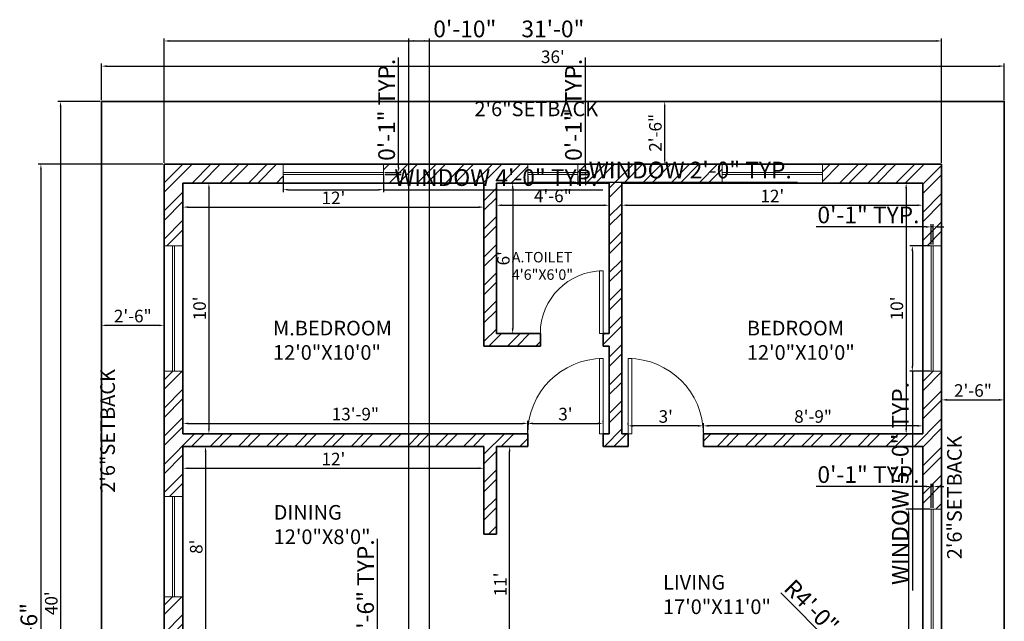
# Model space of a CAD drawing. Units: inches. Extents: x 4732 to 5926, y 2665 to 3255.
# Tile 8 of 8: x 5425 to 5896, y 2967 to 3255. Entities that reach past the tile are written whole.
import ezdxf

# ---------------------------------------------------------------- set-up
doc = ezdxf.new("R2010")
doc.units = ezdxf.units.IN
for name, color, linetype, lineweight in [('A-ANNO-DIMS', 2, 'Continuous', 18), ('A-ANNO-TEXT', 7, 'Continuous', 18), ('A-AREA-IDEN', 7, 'Continuous', 18), ('A-DOOR', 3, 'Continuous', 18), ('A-GLAZ', 4, 'Continuous', 18), ('A-WALL', 7, 'Continuous', 35), ('A-WALL-PATT', 8, 'Continuous', 13), ('C-PROP', 7, 'Continuous', 35)]:
    doc.layers.add(name, color=color, linetype=linetype, lineweight=lineweight)
doc.styles.get("Standard").update_dxf_attribs({"font": 'arial.ttf'})
doc.dimstyles.new('ISO-25', dxfattribs={"dimtxt": 8, "dimasz": 2.5, "dimexe": 1.25, "dimexo": 0.625, "dimtad": 1, "dimdec": 1, "dimlunit": 3, "dimtxsty": 'Standard', "dimcen": 2.5, "dimadec": 0, "dimazin": 0, "dimtfac": 1, "dimtdec": 1, "dimtmove": 0, "dimatfit": 3, "dimfxl": 1, "dimarcsym": 0})

# ---------------------------------------------------------------- blocks, each defined once
blk = doc.blocks.new('*U19')
for p, q in [((0, 0), (0, -6)), ((30, 0), (30, -6))]:
    blk.add_line(p, q)
blk.add_lwpolyline([(0, 0), (0, 30), (1.75, 30), (1.75, 0)], close=True)
blk.add_arc((0, 0), 30, 0, 90)
blk = doc.blocks.new('*U20')
for p, q in [((0, 0), (0, -6)), ((36, 0), (36, -6))]:
    blk.add_line(p, q)
blk.add_lwpolyline([(0, 0), (0, 36), (1.75, 36), (1.75, 0)], close=True)
blk.add_arc((0, 0), 36, 0, 90)
blk = doc.blocks.new('*D29')
at = {"layer": 'A-ANNO-DIMS', "color": 0, "lineweight": -2, "transparency": 16777216}
for p, q in [((5463.94, 3216.56), (5463.94, 3234.09)), ((5466.44, 3232.84), (5893.44, 3232.84)), ((5895.94, 3216.56), (5895.94, 3234.09))]:
    blk.add_line(p, q, dxfattribs=at)
at = {"layer": 'A-ANNO-DIMS', "color": 0, "transparency": 16777216}
for points in [[(5466.44, 3233.25), (5466.44, 3232.42), (5463.94, 3232.84)], [(5893.44, 3233.25), (5893.44, 3232.42), (5895.94, 3232.84)]]:
    blk.add_solid(points, dxfattribs=at)
at = {"layer": 'Defpoints', "color": 0, "transparency": 16777216}
for p in [(5895.94, 3232.84), (5463.94, 3215.93), (5895.94, 3215.93)]:
    blk.add_point(p, dxfattribs=at)
at = {"layer": 'A-ANNO-DIMS', "color": 0, "transparency": 16777216, "insert": (5679.94, 3236.53), "char_height": 6, "attachment_point": 5}
blk.add_mtext("36'", dxfattribs=at)
blk = doc.blocks.new('*D30')
at = {"layer": 'A-ANNO-DIMS', "color": 0, "lineweight": -2, "transparency": 16777216}
for p, q in [((5463.31, 3215.93), (5443.14, 3215.93)), ((5444.39, 3213.43), (5444.39, 2738.43)), ((5463.31, 2735.93), (5443.14, 2735.93))]:
    blk.add_line(p, q, dxfattribs=at)
at = {"layer": 'A-ANNO-DIMS', "color": 0, "transparency": 16777216}
for points in [[(5443.98, 3213.43), (5444.81, 3213.43), (5444.39, 3215.93)], [(5443.98, 2738.43), (5444.81, 2738.43), (5444.39, 2735.93)]]:
    blk.add_solid(points, dxfattribs=at)
at = {"layer": 'Defpoints', "color": 0, "transparency": 16777216}
for p in [(5463.94, 3215.93), (5444.39, 2735.93), (5463.94, 2735.93)]:
    blk.add_point(p, dxfattribs=at)
at = {"layer": 'A-ANNO-DIMS', "color": 0, "transparency": 16777216, "insert": (5440.71, 2975.93), "char_height": 6, "attachment_point": 5, "rotation": 90}
blk.add_mtext("40'", dxfattribs=at)
blk = doc.blocks.new('*D35')
at = {"layer": 'A-ANNO-DIMS', "color": 0, "lineweight": -2, "transparency": 16777216}
for p, q in [((5503.56, 3050.93), (5515.02, 3050.93)), ((5513.77, 3048.43), (5513.77, 2957.43)), ((5503.56, 2954.93), (5515.02, 2954.93))]:
    blk.add_line(p, q, dxfattribs=at)
at = {"layer": 'A-ANNO-DIMS', "color": 0, "transparency": 16777216}
for points in [[(5513.36, 3048.43), (5514.19, 3048.43), (5513.77, 3050.93)], [(5513.36, 2957.43), (5514.19, 2957.43), (5513.77, 2954.93)]]:
    blk.add_solid(points, dxfattribs=at)
at = {"layer": 'Defpoints', "color": 0, "transparency": 16777216}
for p in [(5502.94, 3050.93), (5502.94, 2954.93), (5513.77, 2954.93)]:
    blk.add_point(p, dxfattribs=at)
at = {"layer": 'A-ANNO-DIMS', "color": 0, "transparency": 16777216, "insert": (5510.08, 3002.93), "char_height": 6, "attachment_point": 5, "rotation": 90}
blk.add_mtext("8'", dxfattribs=at)
blk = doc.blocks.new('*D36')
at = {"layer": 'A-ANNO-DIMS', "color": 0, "lineweight": -2, "transparency": 16777216}
for p, q in [((5502.94, 3050.31), (5502.94, 3039.22)), ((5646.94, 3050.31), (5646.94, 3039.22)), ((5505.44, 3040.47), (5644.44, 3040.47))]:
    blk.add_line(p, q, dxfattribs=at)
at = {"layer": 'A-ANNO-DIMS', "color": 0, "transparency": 16777216}
for points in [[(5505.44, 3040.89), (5505.44, 3040.06), (5502.94, 3040.47)], [(5644.44, 3040.89), (5644.44, 3040.06), (5646.94, 3040.47)]]:
    blk.add_solid(points, dxfattribs=at)
at = {"layer": 'Defpoints', "color": 0, "transparency": 16777216}
for p in [(5502.94, 3050.93), (5646.94, 3050.93), (5646.94, 3040.47)]:
    blk.add_point(p, dxfattribs=at)
at = {"layer": 'A-ANNO-DIMS', "color": 0, "transparency": 16777216, "insert": (5574.94, 3044.11), "char_height": 6, "attachment_point": 5}
blk.add_mtext("12'", dxfattribs=at)
blk = doc.blocks.new('*D38')
at = {"layer": 'A-ANNO-DIMS', "color": 0, "lineweight": -2, "transparency": 16777216}
for p, q in [((5653.56, 3050.93), (5660.5, 3050.93)), ((5659.25, 2921.43), (5659.25, 3048.43)), ((5653.56, 2918.93), (5660.5, 2918.93))]:
    blk.add_line(p, q, dxfattribs=at)
at = {"layer": 'A-ANNO-DIMS', "color": 0, "transparency": 16777216}
for points in [[(5658.83, 3048.43), (5659.67, 3048.43), (5659.25, 3050.93)], [(5658.83, 2921.43), (5659.67, 2921.43), (5659.25, 2918.93)]]:
    blk.add_solid(points, dxfattribs=at)
at = {"layer": 'Defpoints', "color": 0, "transparency": 16777216}
for p in [(5652.94, 3050.93), (5659.25, 3050.93), (5652.94, 2918.93)]:
    blk.add_point(p, dxfattribs=at)
at = {"layer": 'A-ANNO-DIMS', "color": 0, "transparency": 16777216, "insert": (5655.61, 2984.93), "char_height": 6, "attachment_point": 5, "rotation": 90}
blk.add_mtext("11'", dxfattribs=at)
blk = doc.blocks.new('*D39')
at = {"layer": 'A-ANNO-DIMS', "color": 0, "lineweight": -2, "transparency": 16777216}
for p, q in [((5712.94, 3176.31), (5712.94, 3165.05)), ((5856.94, 3176.31), (5856.94, 3165.05)), ((5715.44, 3166.3), (5854.44, 3166.3))]:
    blk.add_line(p, q, dxfattribs=at)
at = {"layer": 'A-ANNO-DIMS', "color": 0, "transparency": 16777216}
for points in [[(5715.44, 3166.72), (5715.44, 3165.89), (5712.94, 3166.3)], [(5854.44, 3166.72), (5854.44, 3165.89), (5856.94, 3166.3)]]:
    blk.add_solid(points, dxfattribs=at)
at = {"layer": 'Defpoints', "color": 0, "transparency": 16777216}
for p in [(5712.94, 3176.93), (5856.94, 3176.93), (5856.94, 3166.3)]:
    blk.add_point(p, dxfattribs=at)
at = {"layer": 'A-ANNO-DIMS', "color": 0, "transparency": 16777216, "insert": (5784.94, 3169.94), "char_height": 6, "attachment_point": 5}
blk.add_mtext("12'", dxfattribs=at)
blk = doc.blocks.new('*D40')
at = {"layer": 'A-ANNO-DIMS', "color": 0, "lineweight": -2, "transparency": 16777216}
for p, q in [((5856.31, 3176.93), (5847.73, 3176.93)), ((5848.98, 3174.43), (5848.98, 3059.43)), ((5856.31, 3056.93), (5847.73, 3056.93))]:
    blk.add_line(p, q, dxfattribs=at)
at = {"layer": 'A-ANNO-DIMS', "color": 0, "transparency": 16777216}
for points in [[(5848.56, 3174.43), (5849.4, 3174.43), (5848.98, 3176.93)], [(5848.56, 3059.43), (5849.4, 3059.43), (5848.98, 3056.93)]]:
    blk.add_solid(points, dxfattribs=at)
at = {"layer": 'Defpoints', "color": 0, "transparency": 16777216}
for p in [(5856.94, 3176.93), (5848.98, 3056.93), (5856.94, 3056.93)]:
    blk.add_point(p, dxfattribs=at)
at = {"layer": 'A-ANNO-DIMS', "color": 0, "transparency": 16777216, "insert": (5845.29, 3116.93), "char_height": 6, "attachment_point": 5, "rotation": 90}
blk.add_mtext("10'", dxfattribs=at)
blk = doc.blocks.new('*D41')
at = {"layer": 'A-ANNO-DIMS', "color": 0, "lineweight": -2, "transparency": 16777216}
for p, q in [((5751.94, 3057.56), (5751.94, 3062.02)), ((5854.44, 3060.77), (5754.44, 3060.77)), ((5856.94, 3057.56), (5856.94, 3062.02))]:
    blk.add_line(p, q, dxfattribs=at)
at = {"layer": 'A-ANNO-DIMS', "color": 0, "transparency": 16777216}
for points in [[(5754.44, 3061.19), (5754.44, 3060.35), (5751.94, 3060.77)], [(5854.44, 3061.19), (5854.44, 3060.35), (5856.94, 3060.77)]]:
    blk.add_solid(points, dxfattribs=at)
at = {"layer": 'Defpoints', "color": 0, "transparency": 16777216}
for p in [(5751.94, 3060.77), (5751.94, 3056.93), (5856.94, 3056.93)]:
    blk.add_point(p, dxfattribs=at)
at = {"layer": 'A-ANNO-DIMS', "color": 0, "transparency": 16777216, "insert": (5804.44, 3064.46), "char_height": 6, "attachment_point": 5}
blk.add_mtext('8\'-9"', dxfattribs=at)
blk = doc.blocks.new('*D42')
at = {"layer": 'A-ANNO-DIMS', "color": 0, "lineweight": -2, "transparency": 16777216}
for p, q in [((5715.94, 3061.39), (5715.94, 3062.02)), ((5749.44, 3060.77), (5718.44, 3060.77)), ((5751.94, 3057.56), (5751.94, 3062.02))]:
    blk.add_line(p, q, dxfattribs=at)
at = {"layer": 'A-ANNO-DIMS', "color": 0, "transparency": 16777216}
for points in [[(5718.44, 3061.19), (5718.44, 3060.35), (5715.94, 3060.77)], [(5749.44, 3061.19), (5749.44, 3060.35), (5751.94, 3060.77)]]:
    blk.add_solid(points, dxfattribs=at)
at = {"layer": 'Defpoints', "color": 0, "transparency": 16777216}
for p in [(5715.94, 3060.77), (5715.94, 3060.77), (5751.94, 3056.93)]:
    blk.add_point(p, dxfattribs=at)
at = {"layer": 'A-ANNO-DIMS', "color": 0, "transparency": 16777216, "insert": (5733.94, 3064.46), "char_height": 6, "attachment_point": 5}
blk.add_mtext("3'", dxfattribs=at)
blk = doc.blocks.new('*D43')
at = {"layer": 'A-ANNO-DIMS', "color": 0, "lineweight": -2, "transparency": 16777216}
for p, q in [((5502.94, 3176.31), (5502.94, 3164.15)), ((5646.94, 3176.31), (5646.94, 3164.15)), ((5505.44, 3165.4), (5644.44, 3165.4))]:
    blk.add_line(p, q, dxfattribs=at)
at = {"layer": 'A-ANNO-DIMS', "color": 0, "transparency": 16777216}
for points in [[(5505.44, 3165.81), (5505.44, 3164.98), (5502.94, 3165.4)], [(5644.44, 3165.81), (5644.44, 3164.98), (5646.94, 3165.4)]]:
    blk.add_solid(points, dxfattribs=at)
at = {"layer": 'Defpoints', "color": 0, "transparency": 16777216}
for p in [(5502.94, 3176.93), (5646.94, 3176.93), (5646.94, 3165.4)]:
    blk.add_point(p, dxfattribs=at)
at = {"layer": 'A-ANNO-DIMS', "color": 0, "transparency": 16777216, "insert": (5574.94, 3169.03), "char_height": 6, "attachment_point": 5}
blk.add_mtext("12'", dxfattribs=at)
blk = doc.blocks.new('*D44')
at = {"layer": 'A-ANNO-DIMS', "color": 0, "lineweight": -2, "transparency": 16777216}
for p, q in [((5503.56, 3176.93), (5516.61, 3176.93)), ((5515.36, 3174.43), (5515.36, 3059.43)), ((5503.56, 3056.93), (5516.61, 3056.93))]:
    blk.add_line(p, q, dxfattribs=at)
at = {"layer": 'A-ANNO-DIMS', "color": 0, "transparency": 16777216}
for points in [[(5514.95, 3174.43), (5515.78, 3174.43), (5515.36, 3176.93)], [(5514.95, 3059.43), (5515.78, 3059.43), (5515.36, 3056.93)]]:
    blk.add_solid(points, dxfattribs=at)
at = {"layer": 'Defpoints', "color": 0, "transparency": 16777216}
for p in [(5502.94, 3176.93), (5502.94, 3056.93), (5515.36, 3056.93)]:
    blk.add_point(p, dxfattribs=at)
at = {"layer": 'A-ANNO-DIMS', "color": 0, "transparency": 16777216, "insert": (5511.67, 3116.93), "char_height": 6, "attachment_point": 5, "rotation": 90}
blk.add_mtext("10'", dxfattribs=at)
blk = doc.blocks.new('*D45')
at = {"layer": 'A-ANNO-DIMS', "color": 0, "lineweight": -2, "transparency": 16777216}
for p, q in [((5502.94, 3057.56), (5502.94, 3063.17)), ((5667.94, 3057.56), (5667.94, 3063.17)), ((5505.44, 3061.92), (5665.44, 3061.92))]:
    blk.add_line(p, q, dxfattribs=at)
at = {"layer": 'A-ANNO-DIMS', "color": 0, "transparency": 16777216}
for points in [[(5505.44, 3062.34), (5505.44, 3061.5), (5502.94, 3061.92)], [(5665.44, 3062.34), (5665.44, 3061.5), (5667.94, 3061.92)]]:
    blk.add_solid(points, dxfattribs=at)
at = {"layer": 'Defpoints', "color": 0, "transparency": 16777216}
for p in [(5667.94, 3061.92), (5502.94, 3056.93), (5667.94, 3056.93)]:
    blk.add_point(p, dxfattribs=at)
at = {"layer": 'A-ANNO-DIMS', "color": 0, "transparency": 16777216, "insert": (5585.44, 3065.61), "char_height": 6, "attachment_point": 5}
blk.add_mtext('13\'-9"', dxfattribs=at)
blk = doc.blocks.new('*D46')
at = {"layer": 'A-ANNO-DIMS', "color": 0, "lineweight": -2, "transparency": 16777216}
for p, q in [((5667.94, 3057.56), (5667.94, 3063.17)), ((5703.94, 3062.54), (5703.94, 3063.17)), ((5670.44, 3061.92), (5701.44, 3061.92))]:
    blk.add_line(p, q, dxfattribs=at)
at = {"layer": 'A-ANNO-DIMS', "color": 0, "transparency": 16777216}
for points in [[(5670.44, 3062.34), (5670.44, 3061.5), (5667.94, 3061.92)], [(5701.44, 3062.34), (5701.44, 3061.5), (5703.94, 3061.92)]]:
    blk.add_solid(points, dxfattribs=at)
at = {"layer": 'Defpoints', "color": 0, "transparency": 16777216}
for p in [(5703.94, 3061.92), (5703.94, 3061.92), (5667.94, 3056.93)]:
    blk.add_point(p, dxfattribs=at)
at = {"layer": 'A-ANNO-DIMS', "color": 0, "transparency": 16777216, "insert": (5685.94, 3065.61), "char_height": 6, "attachment_point": 5}
blk.add_mtext("3'", dxfattribs=at)
blk = doc.blocks.new('*D47')
at = {"layer": 'A-ANNO-DIMS', "color": 0, "lineweight": -2, "transparency": 16777216}
for p, q in [((5653.56, 3176.93), (5661.95, 3176.93)), ((5660.7, 3174.43), (5660.7, 3107.43)), ((5653.56, 3104.93), (5661.95, 3104.93))]:
    blk.add_line(p, q, dxfattribs=at)
at = {"layer": 'A-ANNO-DIMS', "color": 0, "transparency": 16777216}
for points in [[(5660.28, 3174.43), (5661.12, 3174.43), (5660.7, 3176.93)], [(5660.28, 3107.43), (5661.12, 3107.43), (5660.7, 3104.93)]]:
    blk.add_solid(points, dxfattribs=at)
at = {"layer": 'Defpoints', "color": 0, "transparency": 16777216}
for p in [(5652.94, 3176.93), (5652.94, 3104.93), (5660.7, 3104.93)]:
    blk.add_point(p, dxfattribs=at)
at = {"layer": 'A-ANNO-DIMS', "color": 0, "transparency": 16777216, "insert": (5657.01, 3140.93), "char_height": 6, "attachment_point": 5, "rotation": 90}
blk.add_mtext("6'", dxfattribs=at)
blk = doc.blocks.new('*D48')
at = {"layer": 'A-ANNO-DIMS', "color": 0, "lineweight": -2, "transparency": 16777216}
for p, q in [((5652.94, 3176.31), (5652.94, 3165.04)), ((5706.94, 3176.31), (5706.94, 3165.04)), ((5655.44, 3166.29), (5704.44, 3166.29))]:
    blk.add_line(p, q, dxfattribs=at)
at = {"layer": 'A-ANNO-DIMS', "color": 0, "transparency": 16777216}
for points in [[(5655.44, 3166.7), (5655.44, 3165.87), (5652.94, 3166.29)], [(5704.44, 3166.7), (5704.44, 3165.87), (5706.94, 3166.29)]]:
    blk.add_solid(points, dxfattribs=at)
at = {"layer": 'Defpoints', "color": 0, "transparency": 16777216}
for p in [(5652.94, 3176.93), (5706.94, 3176.93), (5706.94, 3166.29)]:
    blk.add_point(p, dxfattribs=at)
at = {"layer": 'A-ANNO-DIMS', "color": 0, "transparency": 16777216, "insert": (5679.94, 3169.97), "char_height": 6, "attachment_point": 5}
blk.add_mtext('4\'-6"', dxfattribs=at)
blk = doc.blocks.new('*D49')
at = {"layer": 'A-ANNO-DIMS', "color": 0, "lineweight": -2, "transparency": 16777216}
for p, q in [((5733.45, 3188.43), (5733.45, 3213.43)), ((5734.07, 3215.93), (5734.7, 3215.93)), ((5734.07, 3185.93), (5734.7, 3185.93))]:
    blk.add_line(p, q, dxfattribs=at)
at = {"layer": 'A-ANNO-DIMS', "color": 0, "transparency": 16777216}
for points in [[(5733.03, 3213.43), (5733.86, 3213.43), (5733.45, 3215.93)], [(5733.03, 3188.43), (5733.86, 3188.43), (5733.45, 3185.93)]]:
    blk.add_solid(points, dxfattribs=at)
at = {"layer": 'Defpoints', "color": 0, "transparency": 16777216}
for p in [(5733.45, 3215.93), (5733.45, 3215.93), (5733.45, 3185.93)]:
    blk.add_point(p, dxfattribs=at)
at = {"layer": 'A-ANNO-DIMS', "color": 0, "transparency": 16777216, "insert": (5729.76, 3200.93), "char_height": 6, "attachment_point": 5, "rotation": 90}
blk.add_mtext('2\'-6"', dxfattribs=at)
blk = doc.blocks.new('*D50')
at = {"layer": 'A-ANNO-DIMS', "color": 0, "lineweight": -2, "transparency": 16777216}
for p, q in [((5463.94, 3109.45), (5463.94, 3110.07)), ((5493.94, 3109.45), (5493.94, 3110.07)), ((5491.44, 3108.82), (5466.44, 3108.82))]:
    blk.add_line(p, q, dxfattribs=at)
at = {"layer": 'A-ANNO-DIMS', "color": 0, "transparency": 16777216}
for points in [[(5466.44, 3109.24), (5466.44, 3108.41), (5463.94, 3108.82)], [(5491.44, 3109.24), (5491.44, 3108.41), (5493.94, 3108.82)]]:
    blk.add_solid(points, dxfattribs=at)
at = {"layer": 'Defpoints', "color": 0, "transparency": 16777216}
for p in [(5463.94, 3108.82), (5463.94, 3108.82), (5493.94, 3108.82)]:
    blk.add_point(p, dxfattribs=at)
at = {"layer": 'A-ANNO-DIMS', "color": 0, "transparency": 16777216, "insert": (5478.94, 3112.51), "char_height": 6, "attachment_point": 5}
blk.add_mtext('2\'-6"', dxfattribs=at)
blk = doc.blocks.new('*D51')
at = {"layer": 'A-ANNO-DIMS', "color": 0, "lineweight": -2, "transparency": 16777216}
for p, q in [((5865.94, 3073.82), (5865.94, 3074.44)), ((5868.44, 3073.19), (5893.44, 3073.19)), ((5895.94, 3073.82), (5895.94, 3074.44))]:
    blk.add_line(p, q, dxfattribs=at)
at = {"layer": 'A-ANNO-DIMS', "color": 0, "transparency": 16777216}
for points in [[(5868.44, 3073.61), (5868.44, 3072.78), (5865.94, 3073.19)], [(5893.44, 3073.61), (5893.44, 3072.78), (5895.94, 3073.19)]]:
    blk.add_solid(points, dxfattribs=at)
at = {"layer": 'Defpoints', "color": 0, "transparency": 16777216}
for p in [(5865.94, 3073.19), (5895.94, 3073.19), (5895.94, 3073.19)]:
    blk.add_point(p, dxfattribs=at)
at = {"layer": 'A-ANNO-DIMS', "color": 0, "transparency": 16777216, "insert": (5880.94, 3076.88), "char_height": 6, "attachment_point": 5}
blk.add_mtext('2\'-6"', dxfattribs=at)
blk = doc.blocks.new('GLAZ-UNIT-48IN')
for p, q in [((0, 1), (48, 1)), ((0, 0), (48, 0))]:
    blk.add_line(p, q)
blk = doc.blocks.new('GLAZ-UNIT-60IN')
for p, q in [((0, 0), (0, 60)), ((1, 0), (1, 60))]:
    blk.add_line(p, q)
blk = doc.blocks.new('GLAZ-UNIT-24IN')
for p, q in [((0, 1), (24, 1)), ((0, 0), (24, 0))]:
    blk.add_line(p, q)
blk = doc.blocks.new('GLAZ-UNIT-72IN')
for p, q in [((0, 72), (0, 0)), ((1, 72), (1, 0))]:
    blk.add_line(p, q)
blk = doc.blocks.new('*D62')
at = {"layer": 'A-ANNO-DIMS', "color": 0, "lineweight": -2, "transparency": 16777216}
for p, q in [((5550.94, 3180.31), (5550.94, 3172.48)), ((5598.94, 3180.31), (5598.94, 3172.48)), ((5553.44, 3173.73), (5596.44, 3173.73)), ((5598.94, 3173.73), (5703.92, 3173.73))]:
    blk.add_line(p, q, dxfattribs=at)
at = {"layer": 'A-ANNO-DIMS', "color": 0, "transparency": 16777216}
for points in [[(5553.44, 3174.15), (5553.44, 3173.32), (5550.94, 3173.73)], [(5596.44, 3174.15), (5596.44, 3173.32), (5598.94, 3173.73)]]:
    blk.add_solid(points, dxfattribs=at)
at = {"layer": 'Defpoints', "color": 0, "transparency": 16777216}
for p in [(5550.94, 3180.93), (5598.94, 3180.93), (5598.94, 3173.73)]:
    blk.add_point(p, dxfattribs=at)
at = {"layer": 'A-ANNO-DIMS', "color": 0, "transparency": 16777216, "insert": (5652.68, 3178.5), "char_height": 8, "attachment_point": 5}
blk.add_mtext('WINDOW 4\'-0" TYP.', dxfattribs=at)
blk = doc.blocks.new('*D63')
at = {"layer": 'A-ANNO-DIMS', "color": 0, "lineweight": -2, "transparency": 16777216}
for p, q in [((5606.14, 3184.43), (5606.14, 3236.95)), ((5599.56, 3181.93), (5607.39, 3181.93)), ((5599.56, 3180.93), (5607.39, 3180.93)), ((5606.14, 3180.93), (5606.14, 3181.93)), ((5606.14, 3178.43), (5606.14, 3175.93))]:
    blk.add_line(p, q, dxfattribs=at)
at = {"layer": 'A-ANNO-DIMS', "color": 0, "transparency": 16777216}
for points in [[(5605.72, 3184.43), (5606.55, 3184.43), (5606.14, 3181.93)], [(5605.72, 3178.43), (5606.55, 3178.43), (5606.14, 3180.93)]]:
    blk.add_solid(points, dxfattribs=at)
at = {"layer": 'Defpoints', "color": 0, "transparency": 16777216}
for p in [(5598.94, 3181.93), (5598.94, 3180.93), (5606.14, 3181.93)]:
    blk.add_point(p, dxfattribs=at)
at = {"layer": 'A-ANNO-DIMS', "color": 0, "transparency": 16777216, "insert": (5601.43, 3211.94), "char_height": 8, "attachment_point": 5, "rotation": 90}
blk.add_mtext('0\'-1" TYP.', dxfattribs=at)
blk = doc.blocks.new('*D64')
at = {"layer": 'A-ANNO-DIMS', "color": 0, "lineweight": -2, "transparency": 16777216}
for p, q in [((5860.31, 3146.93), (5850.69, 3146.93)), ((5851.94, 3144.43), (5851.94, 3089.43)), ((5860.31, 3086.93), (5850.69, 3086.93)), ((5851.94, 3086.93), (5851.94, 2981.95))]:
    blk.add_line(p, q, dxfattribs=at)
at = {"layer": 'A-ANNO-DIMS', "color": 0, "transparency": 16777216}
for points in [[(5851.52, 3144.43), (5852.35, 3144.43), (5851.94, 3146.93)], [(5851.52, 3089.43), (5852.35, 3089.43), (5851.94, 3086.93)]]:
    blk.add_solid(points, dxfattribs=at)
at = {"layer": 'Defpoints', "color": 0, "transparency": 16777216}
for p in [(5860.94, 3146.93), (5851.94, 3086.93), (5860.94, 3086.93)]:
    blk.add_point(p, dxfattribs=at)
at = {"layer": 'A-ANNO-DIMS', "color": 0, "transparency": 16777216, "insert": (5847.17, 3033.19), "char_height": 8, "attachment_point": 5, "rotation": 90}
blk.add_mtext('WINDOW 5\'-0" TYP.', dxfattribs=at)
blk = doc.blocks.new('*D65')
at = {"layer": 'A-ANNO-DIMS', "color": 0, "lineweight": -2, "transparency": 16777216}
for p, q in [((5860.94, 3147.56), (5860.94, 3157.18)), ((5861.94, 3147.56), (5861.94, 3157.18)), ((5858.44, 3155.93), (5805.92, 3155.93)), ((5861.94, 3155.93), (5860.94, 3155.93)), ((5864.44, 3155.93), (5866.94, 3155.93))]:
    blk.add_line(p, q, dxfattribs=at)
at = {"layer": 'A-ANNO-DIMS', "color": 0, "transparency": 16777216}
for points in [[(5858.44, 3156.35), (5858.44, 3155.52), (5860.94, 3155.93)], [(5864.44, 3156.35), (5864.44, 3155.52), (5861.94, 3155.93)]]:
    blk.add_solid(points, dxfattribs=at)
at = {"layer": 'Defpoints', "color": 0, "transparency": 16777216}
for p in [(5860.94, 3155.93), (5860.94, 3146.93), (5861.94, 3146.93)]:
    blk.add_point(p, dxfattribs=at)
at = {"layer": 'A-ANNO-DIMS', "color": 0, "transparency": 16777216, "insert": (5830.93, 3160.64), "char_height": 8, "attachment_point": 5}
blk.add_mtext('0\'-1" TYP.', dxfattribs=at)
blk = doc.blocks.new('*D66')
at = {"layer": 'A-ANNO-DIMS', "color": 0, "lineweight": -2, "transparency": 16777216}
for p, q in [((5667.94, 3180.31), (5667.94, 3176.08)), ((5691.94, 3180.31), (5691.94, 3176.08)), ((5670.44, 3177.33), (5689.44, 3177.33)), ((5691.94, 3177.33), (5796.92, 3177.33))]:
    blk.add_line(p, q, dxfattribs=at)
at = {"layer": 'A-ANNO-DIMS', "color": 0, "transparency": 16777216}
for points in [[(5670.44, 3177.75), (5670.44, 3176.92), (5667.94, 3177.33)], [(5689.44, 3177.75), (5689.44, 3176.92), (5691.94, 3177.33)]]:
    blk.add_solid(points, dxfattribs=at)
at = {"layer": 'Defpoints', "color": 0, "transparency": 16777216}
for p in [(5667.94, 3180.93), (5691.94, 3180.93), (5691.94, 3177.33)]:
    blk.add_point(p, dxfattribs=at)
at = {"layer": 'A-ANNO-DIMS', "color": 0, "transparency": 16777216, "insert": (5745.68, 3182.1), "char_height": 8, "attachment_point": 5}
blk.add_mtext('WINDOW 2\'-0" TYP.', dxfattribs=at)
blk = doc.blocks.new('*D67')
at = {"layer": 'A-ANNO-DIMS', "color": 0, "lineweight": -2, "transparency": 16777216}
for p, q in [((5695.54, 3184.43), (5695.54, 3236.95)), ((5692.56, 3181.93), (5696.79, 3181.93)), ((5692.56, 3180.93), (5696.79, 3180.93)), ((5695.54, 3180.93), (5695.54, 3181.93)), ((5695.54, 3178.43), (5695.54, 3175.93))]:
    blk.add_line(p, q, dxfattribs=at)
at = {"layer": 'A-ANNO-DIMS', "color": 0, "transparency": 16777216}
for points in [[(5695.12, 3184.43), (5695.95, 3184.43), (5695.54, 3181.93)], [(5695.12, 3178.43), (5695.95, 3178.43), (5695.54, 3180.93)]]:
    blk.add_solid(points, dxfattribs=at)
at = {"layer": 'Defpoints', "color": 0, "transparency": 16777216}
for p in [(5691.94, 3181.93), (5691.94, 3180.93), (5695.54, 3181.93)]:
    blk.add_point(p, dxfattribs=at)
at = {"layer": 'A-ANNO-DIMS', "color": 0, "transparency": 16777216, "insert": (5690.83, 3211.94), "char_height": 8, "attachment_point": 5, "rotation": 90}
blk.add_mtext('0\'-1" TYP.', dxfattribs=at)
blk = doc.blocks.new('*D68')
at = {"layer": 'A-ANNO-DIMS', "color": 0, "lineweight": -2, "transparency": 16777216}
for p, q in [((5860.31, 3020.93), (5848.89, 3020.93)), ((5850.14, 3018.43), (5850.14, 2951.43)), ((5860.31, 2948.93), (5848.89, 2948.93)), ((5850.14, 2948.93), (5850.14, 2843.95))]:
    blk.add_line(p, q, dxfattribs=at)
at = {"layer": 'A-ANNO-DIMS', "color": 0, "transparency": 16777216}
for points in [[(5849.72, 3018.43), (5850.55, 3018.43), (5850.14, 3020.93)], [(5849.72, 2951.43), (5850.55, 2951.43), (5850.14, 2948.93)]]:
    blk.add_solid(points, dxfattribs=at)
at = {"layer": 'Defpoints', "color": 0, "transparency": 16777216}
for p in [(5860.94, 3020.93), (5850.14, 2948.93), (5860.94, 2948.93)]:
    blk.add_point(p, dxfattribs=at)
at = {"layer": 'A-ANNO-DIMS', "color": 0, "transparency": 16777216, "insert": (5845.37, 2895.19), "char_height": 8, "attachment_point": 5, "rotation": 90}
blk.add_mtext('WINDOW 6\'-0" TYP.', dxfattribs=at)
blk = doc.blocks.new('*D69')
at = {"layer": 'A-ANNO-DIMS', "color": 0, "lineweight": -2, "transparency": 16777216}
for p, q in [((5858.44, 3031.73), (5805.92, 3031.73)), ((5860.94, 3021.56), (5860.94, 3032.98)), ((5861.94, 3031.73), (5860.94, 3031.73)), ((5861.94, 3021.56), (5861.94, 3032.98)), ((5864.44, 3031.73), (5866.94, 3031.73))]:
    blk.add_line(p, q, dxfattribs=at)
at = {"layer": 'A-ANNO-DIMS', "color": 0, "transparency": 16777216}
for points in [[(5858.44, 3032.15), (5858.44, 3031.32), (5860.94, 3031.73)], [(5864.44, 3032.15), (5864.44, 3031.32), (5861.94, 3031.73)]]:
    blk.add_solid(points, dxfattribs=at)
at = {"layer": 'Defpoints', "color": 0, "transparency": 16777216}
for p in [(5860.94, 3031.73), (5860.94, 3020.93), (5861.94, 3020.93)]:
    blk.add_point(p, dxfattribs=at)
at = {"layer": 'A-ANNO-DIMS', "color": 0, "transparency": 16777216, "insert": (5830.93, 3036.44), "char_height": 8, "attachment_point": 5}
blk.add_mtext('0\'-1" TYP.', dxfattribs=at)
blk = doc.blocks.new('*D73')
at = {"layer": 'A-ANNO-DIMS', "color": 0, "lineweight": -2, "transparency": 16777216}
for p, q in [((5596.05, 2954.93), (5596.05, 3006.69)), ((5587.66, 2954.93), (5597.3, 2954.93)), ((5596.05, 2939.43), (5596.05, 2952.43)), ((5587.66, 2936.93), (5597.3, 2936.93))]:
    blk.add_line(p, q, dxfattribs=at)
at = {"layer": 'A-ANNO-DIMS', "color": 0, "transparency": 16777216}
for points in [[(5595.64, 2952.43), (5596.47, 2952.43), (5596.05, 2954.93)], [(5595.64, 2939.43), (5596.47, 2939.43), (5596.05, 2936.93)]]:
    blk.add_solid(points, dxfattribs=at)
at = {"layer": 'Defpoints', "color": 0, "transparency": 16777216}
for p in [(5587.04, 2954.93), (5596.05, 2954.93), (5587.04, 2936.93)]:
    blk.add_point(p, dxfattribs=at)
at = {"layer": 'A-ANNO-DIMS', "color": 0, "transparency": 16777216, "insert": (5591.34, 2982.06), "char_height": 8, "attachment_point": 5, "rotation": 90}
blk.add_mtext('1\'-6" TYP.', dxfattribs=at)
blk = doc.blocks.new('*D104')
at = {"layer": 'A-ANNO-DIMS', "color": 0, "lineweight": -2, "transparency": 16777216}
for p, q in [((5493.94, 3186.56), (5493.94, 3246.13)), ((5865.94, 3186.56), (5865.94, 3246.13)), ((5496.44, 3244.88), (5863.44, 3244.88))]:
    blk.add_line(p, q, dxfattribs=at)
at = {"layer": 'A-ANNO-DIMS', "color": 0, "transparency": 16777216}
for points in [[(5496.44, 3245.3), (5496.44, 3244.47), (5493.94, 3244.88)], [(5863.44, 3245.3), (5863.44, 3244.47), (5865.94, 3244.88)]]:
    blk.add_solid(points, dxfattribs=at)
at = {"layer": 'Defpoints', "color": 0, "transparency": 16777216}
for p in [(5865.94, 3244.88), (5493.94, 3185.93), (5865.94, 3185.93)]:
    blk.add_point(p, dxfattribs=at)
at = {"layer": 'A-ANNO-DIMS', "color": 0, "transparency": 16777216, "insert": (5679.94, 3249.6), "char_height": 8, "attachment_point": 5}
blk.add_mtext('31\'-0"', dxfattribs=at)
blk = doc.blocks.new('*D105')
at = {"layer": 'A-ANNO-DIMS', "color": 0, "lineweight": -2, "transparency": 16777216}
for p, q in [((5493.31, 3185.93), (5433.74, 3185.93)), ((5434.99, 3183.43), (5434.99, 2738.43)), ((5493.31, 2735.93), (5433.74, 2735.93))]:
    blk.add_line(p, q, dxfattribs=at)
at = {"layer": 'A-ANNO-DIMS', "color": 0, "transparency": 16777216}
for points in [[(5434.57, 3183.43), (5435.4, 3183.43), (5434.99, 3185.93)], [(5434.57, 2738.43), (5435.4, 2738.43), (5434.99, 2735.93)]]:
    blk.add_solid(points, dxfattribs=at)
at = {"layer": 'Defpoints', "color": 0, "transparency": 16777216}
for p in [(5493.94, 3185.93), (5434.99, 2735.93), (5493.94, 2735.93)]:
    blk.add_point(p, dxfattribs=at)
at = {"layer": 'A-ANNO-DIMS', "color": 0, "transparency": 16777216, "insert": (5430.27, 2960.93), "char_height": 8, "attachment_point": 5, "rotation": 90}
blk.add_mtext('37\'-6"', dxfattribs=at)
blk = doc.blocks.new('*D111')
at = {"layer": 'A-ANNO-DIMS', "color": 0, "lineweight": -2, "transparency": 16777216}
for p, q in [((5610.94, 2817.56), (5610.94, 3246.13)), ((5620.94, 2817.56), (5620.94, 3246.13)), ((5613.44, 3244.88), (5618.44, 3244.88)), ((5620.94, 3244.88), (5652.17, 3244.88))]:
    blk.add_line(p, q, dxfattribs=at)
at = {"layer": 'A-ANNO-DIMS', "color": 0, "transparency": 16777216}
for points in [[(5613.44, 3245.3), (5613.44, 3244.47), (5610.94, 3244.88)], [(5618.44, 3245.3), (5618.44, 3244.47), (5620.94, 3244.88)]]:
    blk.add_solid(points, dxfattribs=at)
at = {"layer": 'Defpoints', "color": 0, "transparency": 16777216}
for p in [(5620.94, 3244.88), (5610.94, 2816.93), (5620.94, 2816.93)]:
    blk.add_point(p, dxfattribs=at)
at = {"layer": 'A-ANNO-DIMS', "color": 0, "transparency": 16777216, "insert": (5637.8, 3249.59), "char_height": 8, "attachment_point": 5}
blk.add_mtext('0\'-10"', dxfattribs=at)
blk = doc.blocks.new('*D117')
at = {"layer": 'A-ANNO-DIMS', "color": 0, "lineweight": -2, "transparency": 16777216}
for p, q in [((5788.96, 2980.91), (5818.23, 2951.64)), ((5853.94, 2915.93), (5820, 2949.87))]:
    blk.add_line(p, q, dxfattribs=at)
at = {"layer": 'A-ANNO-DIMS', "color": 0, "transparency": 16777216}
blk.add_solid([(5818.52, 2951.94), (5817.93, 2951.35), (5820, 2949.87)], dxfattribs=at)
at = {"layer": 'Defpoints', "color": 0, "transparency": 16777216}
for p in [(5820, 2949.87), (5853.94, 2915.93)]:
    blk.add_point(p, dxfattribs=at)
at = {"layer": 'A-ANNO-DIMS', "color": 0, "transparency": 16777216, "insert": (5802.96, 2973.57), "char_height": 8, "attachment_point": 5, "rotation": 315.0001}
blk.add_mtext('R4\'-0"', dxfattribs=at)

msp = doc.modelspace()

# ---------------------------------------------------------------- hatches: boundary and pattern name
at = {"layer": 'A-WALL-PATT'}
h = msp.add_hatch(dxfattribs=at)
h.set_pattern_fill('ANSI32', color=256)
h.paths.add_polyline_path([(5502.94, 3086.93), (5493.94, 3086.93), (5493.94, 3026.93), (5502.94, 3026.93), (5502.94, 3050.93), (5646.94, 3050.93), (5646.94, 3008.93), (5652.94, 3008.93), (5652.94, 3050.93), (5667.94, 3050.93), (5667.94, 3056.93), (5502.94, 3056.93)])
h.paths.add_polyline_path([(5502.94, 2978.93), (5493.94, 2978.93), (5493.94, 2945.93), (5517.94, 2945.93), (5517.94, 2933.93), (5520.94, 2933.93), (5526.94, 2933.93), (5526.94, 2954.93), (5502.94, 2954.93)])
h.paths.add_polyline_path([(5526.94, 2849.93), (5517.94, 2849.93), (5517.94, 2825.93), (5493.94, 2825.93), (5493.94, 2804.93), (5502.94, 2804.93), (5502.94, 2816.93), (5574.94, 2816.93), (5574.94, 2825.93), (5526.94, 2825.93)])
h.paths.add_polyline_path([(5526.94, 2903.93), (5520.94, 2903.93), (5517.94, 2903.93), (5517.94, 2897.93), (5526.94, 2897.93)])
h.paths.add_polyline_path([(5655.94, 2909.93), (5805.94, 2909.93), (5805.94, 2915.93), (5805.94, 2918.93), (5652.94, 2918.93), (5652.94, 2960.93), (5646.94, 2960.93), (5646.94, 2825.93), (5622.94, 2825.93), (5622.94, 2816.93), (5655.94, 2816.93)])
h.paths.add_polyline_path([(5620.94, 2744.93), (5502.94, 2744.93), (5502.94, 2756.93), (5493.94, 2756.93), (5493.94, 2735.93), (5620.94, 2735.93)])
h.paths.add_polyline_path([(5865.94, 2948.93), (5856.94, 2948.93), (5856.94, 2918.93), (5853.94, 2918.93), (5853.94, 2915.93), (5853.94, 2909.93), (5865.94, 2909.93)])
h.paths.add_polyline_path([(5865.94, 3086.93), (5856.94, 3086.93), (5856.94, 3056.93), (5751.94, 3056.93), (5751.94, 3050.93), (5856.94, 3050.93), (5856.94, 3020.93), (5865.94, 3020.93)])
h.paths.add_polyline_path([(5865.94, 3185.93), (5808.94, 3185.93), (5808.94, 3176.93), (5856.94, 3176.93), (5856.94, 3146.93), (5865.94, 3146.93)])
h.paths.add_polyline_path([(5760.94, 3185.93), (5691.94, 3185.93), (5691.94, 3176.93), (5706.94, 3176.93), (5706.94, 3104.93), (5703.94, 3104.93), (5703.94, 3098.93), (5706.94, 3098.93), (5706.94, 3056.93), (5703.94, 3056.93), (5703.94, 3050.93), (5706.94, 3050.93), (5715.94, 3050.93), (5715.94, 3056.93), (5712.94, 3056.93), (5712.94, 3176.93), (5760.94, 3176.93)])
h.paths.add_polyline_path([(5667.94, 3185.93), (5598.94, 3185.93), (5598.94, 3176.93), (5646.94, 3176.93), (5646.94, 3098.93), (5673.94, 3098.93), (5673.94, 3104.93), (5652.94, 3104.93), (5652.94, 3176.93), (5667.94, 3176.93)])
h.paths.add_polyline_path([(5550.94, 3185.93), (5493.94, 3185.93), (5493.94, 3146.93), (5502.94, 3146.93), (5502.94, 3176.93), (5550.94, 3176.93)])

# ---------------------------------------------------------------- linework, layer by layer
at = {"layer": 'A-GLAZ'}
for p, q in [((5550.94, 3176.93), (5550.94, 3185.93)), ((5598.94, 3176.93), (5598.94, 3185.93)), ((5667.94, 3176.93), (5667.94, 3185.93)), ((5691.94, 3176.93), (5691.94, 3185.93)), ((5760.94, 3176.93), (5760.94, 3185.93)), ((5808.94, 3176.93), (5808.94, 3185.93)), ((5502.94, 3146.93), (5493.94, 3146.93)), ((5856.94, 3146.93), (5865.94, 3146.93)), ((5502.94, 3086.93), (5493.94, 3086.93)), ((5856.94, 3086.93), (5865.94, 3086.93)), ((5502.94, 3026.93), (5493.94, 3026.93)), ((5856.94, 3020.93), (5865.94, 3020.93)), ((5502.94, 2978.93), (5493.94, 2978.93))]:
    msp.add_line(p, q, dxfattribs=at)
at = {"layer": 'A-WALL'}
for p, q in [((5493.94, 3185.93), (5865.94, 3185.93)), ((5493.94, 2945.93), (5493.94, 3185.93)), ((5865.94, 3185.93), (5865.94, 2885.93)), ((5502.94, 3176.93), (5646.94, 3176.93)), ((5502.94, 3056.93), (5502.94, 3176.93)), ((5646.94, 3098.93), (5646.94, 3176.93)), ((5652.94, 3176.93), (5706.94, 3176.93)), ((5652.94, 3104.93), (5652.94, 3176.93)), ((5706.94, 3176.93), (5706.94, 3104.93)), ((5712.94, 3176.93), (5856.94, 3176.93)), ((5712.94, 3176.93), (5712.94, 3056.93)), ((5856.94, 3176.93), (5856.94, 3056.93)), ((5652.94, 3104.93), (5673.94, 3104.93)), ((5673.94, 3104.93), (5673.94, 3098.93)), ((5703.94, 3104.93), (5706.94, 3104.93)), ((5703.94, 3104.93), (5703.94, 3098.93)), ((5646.94, 3098.93), (5673.94, 3098.93)), ((5703.94, 3098.93), (5706.94, 3098.93)), ((5706.94, 3098.93), (5706.94, 3056.93)), ((5502.94, 3056.93), (5667.94, 3056.93)), ((5667.94, 3056.93), (5667.94, 3050.93)), ((5703.94, 3056.93), (5706.94, 3056.93)), ((5703.94, 3056.93), (5703.94, 3050.93)), ((5712.94, 3056.93), (5715.94, 3056.93)), ((5715.94, 3056.93), (5715.94, 3050.93)), ((5751.94, 3056.93), (5856.94, 3056.93)), ((5751.94, 3056.93), (5751.94, 3050.93)), ((5502.94, 3050.93), (5646.94, 3050.93)), ((5502.94, 2954.93), (5502.94, 3050.93)), ((5646.94, 3008.93), (5646.94, 3050.93)), ((5652.94, 3050.93), (5667.94, 3050.93)), ((5652.94, 3008.93), (5652.94, 3050.93)), ((5703.94, 3050.93), (5706.94, 3050.93)), ((5706.94, 3050.93), (5715.94, 3050.93)), ((5751.94, 3050.93), (5856.94, 3050.93)), ((5856.94, 3050.93), (5856.94, 2918.93)), ((5646.94, 3008.93), (5652.94, 3008.93))]:
    msp.add_line(p, q, dxfattribs=at)
at = {"layer": 'C-PROP'}
msp.add_lwpolyline([(5463.94, 3215.93), (5895.94, 3215.93), (5895.94, 2735.93), (5463.94, 2735.93)], close=True, dxfattribs=at)

# ---------------------------------------------------------------- block references
at = {"layer": 'A-DOOR', "xscale": -1}
for name, p in [('*U19', (5703.94, 3104.93)), ('*U20', (5703.94, 3056.93))]:
    msp.add_blockref(name, p, dxfattribs=at)
at = {"layer": 'A-DOOR'}
msp.add_blockref('*U20', (5715.94, 3056.93), dxfattribs=at)
at = {"layer": 'A-GLAZ'}
for name, p in [('GLAZ-UNIT-48IN', (5550.94, 3180.93)), ('GLAZ-UNIT-24IN', (5667.94, 3180.93)), ('GLAZ-UNIT-48IN', (5760.94, 3180.93)), ('GLAZ-UNIT-60IN', (5497.94, 3086.93))]:
    msp.add_blockref(name, p, dxfattribs=at)
for name, p, rotation in [('GLAZ-UNIT-60IN', (5861.94, 3146.93), 180), ('GLAZ-UNIT-48IN', (5497.94, 3026.93), 270), ('GLAZ-UNIT-72IN', (5861.94, 3020.93), 180)]:
    msp.add_blockref(name, p, dxfattribs=dict(at, rotation=rotation))

# ---------------------------------------------------------------- texts
at = {"layer": 'A-ANNO-TEXT', "insert": (5642.42, 3215.89), "char_height": 7, "attachment_point": 1}
msp.add_mtext_dynamic_manual_height_columns('{\\fTimes New Roman|b0|i0|c0|p18; 2\'6"SETBACK }', width=61.0557, gutter_width=12.5, heights=[0], dxfattribs=at)
at = {"layer": 'A-ANNO-TEXT', "char_height": 7, "attachment_point": 1, "rotation": 90}
for insert in [(5463.39, 3028.76), (5868.56, 2996.95)]:
    msp.add_mtext_dynamic_manual_height_columns('{\\fTimes New Roman|b0|i0|c0|p18; 2\'6"SETBACK }', width=61.0557, gutter_width=12.5, heights=[0], dxfattribs=dict(at, insert=insert))
at = {"layer": 'A-AREA-IDEN', "attachment_point": 1}
for s, insert, char_height in [('{\\fTimes New Roman|b0|i0|c0|p18;A.TOILET\\P4\'6"X6\'0"}', (5660.28, 3143.95), 5), ('{\\fTimes New Roman|b0|i0|c0|p18;M.BEDROOM\\P12\'0"X10\'0"}', (5546.03, 3111.03), 7), ('{\\fTimes New Roman|b0|i0|c0|p18;BEDROOM\\P12\'0"X10\'0"}', (5772.76, 3111.03), 7), ('{\\fTimes New Roman|b0|i0|c0|p18;DINING\\P12\'0"X8\'0"}', (5546.36, 3022.89), 7), ('{\\fTimes New Roman|b0|i0|c0|p18;LIVING 17\'0"X11\'0"}', (5732.63, 2989.4), 7)]:
    msp.add_mtext_dynamic_manual_height_columns(s, width=61.0557, gutter_width=12.5, heights=[0], dxfattribs=dict(at, insert=insert, char_height=char_height))

# ---------------------------------------------------------------- dimensions: what is measured, and where the dimension line sits
at = {"layer": 'A-ANNO-DIMS'}
for base, p1, p2, override, picture, middle in [((5865.94, 3244.88), (5493.94, 3185.93), (5865.94, 3185.93), {"dimdec": 1, "dimlfac": 1, "dimrnd": 0, "dimzin": 1, "dimdsep": 46, "dimlunit": 4, "dimfrac": 2}, '*D104', (5679.94, 3249.6)), ((5620.94, 3244.88), (5610.94, 2816.93), (5620.94, 2816.93), {"dimdec": 1, "dimlfac": 1, "dimrnd": 0, "dimzin": 1, "dimdsep": 46, "dimlunit": 4, "dimfrac": 2}, '*D111', (5637.8, 3249.59)), ((5895.94, 3232.84), (5463.94, 3215.93), (5895.94, 3215.93), {"dimtxt": 6, "dimclrd": 0, "dimclre": 0, "dimclrt": 0}, '*D29', (5679.94, 3236.53)), ((5646.94, 3165.4), (5502.94, 3176.93), (5646.94, 3176.93), {"dimtxt": 6, "dimclrd": 0, "dimclre": 0, "dimclrt": 0}, '*D43', (5574.94, 3169.03)), ((5706.94, 3166.29), (5652.94, 3176.93), (5706.94, 3176.93), {"dimtxt": 6, "dimclrd": 0, "dimclre": 0, "dimclrt": 0}, '*D48', (5679.94, 3169.97)), ((5856.94, 3166.3), (5712.94, 3176.93), (5856.94, 3176.93), {"dimtxt": 6, "dimclrd": 0, "dimclre": 0, "dimclrt": 0}, '*D39', (5784.94, 3169.94)), ((5463.94, 3108.82), (5493.94, 3108.82), (5463.94, 3108.82), {"dimtxt": 6, "dimclrd": 0, "dimclre": 0, "dimclrt": 0}, '*D50', (5478.94, 3112.51)), ((5895.94, 3073.19), (5865.94, 3073.19), (5895.94, 3073.19), {"dimtxt": 6, "dimclrd": 0, "dimclre": 0, "dimclrt": 0}, '*D51', (5880.94, 3076.88)), ((5667.94, 3061.92), (5502.94, 3056.93), (5667.94, 3056.93), {"dimtxt": 6, "dimclrd": 0, "dimclre": 0, "dimclrt": 0}, '*D45', (5585.44, 3065.61)), ((5703.94, 3061.92), (5667.94, 3056.93), (5703.94, 3061.92), {"dimtxt": 6, "dimclrd": 0, "dimclre": 0, "dimclrt": 0, "dimtmove": 1}, '*D46', (5685.94, 3065.61)), ((5715.94, 3060.77), (5751.94, 3056.93), (5715.94, 3060.77), {"dimtxt": 6, "dimclrd": 0, "dimclre": 0, "dimclrt": 0, "dimtmove": 1}, '*D42', (5733.94, 3064.46)), ((5751.94, 3060.77), (5856.94, 3056.93), (5751.94, 3056.93), {"dimtxt": 6, "dimclrd": 0, "dimclre": 0, "dimclrt": 0}, '*D41', (5804.44, 3064.46)), ((5646.94, 3040.47), (5502.94, 3050.93), (5646.94, 3050.93), {"dimtxt": 6, "dimclrd": 0, "dimclre": 0, "dimclrt": 0}, '*D36', (5574.94, 3044.11))]:
    dim = msp.add_linear_dim(base=base, p1=p1, p2=p2, dimstyle='ISO-25', override=override, dxfattribs=at)
    dim.commit()
    dim.dimension.update_dxf_attribs({"geometry": picture, "text_midpoint": middle})
for base, p1, p2, angle, text, picture, middle in [((5606.14, 3181.93), (5598.94, 3180.93), (5598.94, 3181.93), 90, '<> TYP.', '*D63', (5601.43, 3211.94)), ((5695.54, 3181.93), (5691.94, 3180.93), (5691.94, 3181.93), 90, '<> TYP.', '*D67', (5690.83, 3211.94)), ((5860.94, 3155.93), (5861.94, 3146.93), (5860.94, 3146.93), 180, '<> TYP.', '*D65', (5830.93, 3160.64)), ((5851.94, 3086.93), (5860.94, 3146.93), (5860.94, 3086.93), 270, 'WINDOW <> TYP.', '*D64', (5847.17, 3033.19)), ((5860.94, 3031.73), (5861.94, 3020.93), (5860.94, 3020.93), 180, '<> TYP.', '*D69', (5830.93, 3036.44)), ((5850.14, 2948.93), (5860.94, 3020.93), (5860.94, 2948.93), 270, 'WINDOW <> TYP.', '*D68', (5845.37, 2895.19)), ((5596.05, 2954.93), (5587.04, 2936.93), (5587.04, 2954.93), 90, '<> TYP.', '*D73', (5591.34, 2982.06))]:
    dim = msp.add_linear_dim(base=base, p1=p1, p2=p2, angle=angle, text=text, dimstyle='ISO-25', override={"dimdec": 1, "dimlfac": 1, "dimrnd": 0, "dimzin": 1, "dimdsep": 46, "dimlunit": 4, "dimfrac": 2}, dxfattribs=at)
    dim.commit()
    dim.dimension.update_dxf_attribs({"geometry": picture, "text_midpoint": middle})
for base, p1, p2, override, picture, middle in [((5444.39, 2735.93), (5463.94, 3215.93), (5463.94, 2735.93), {"dimtxt": 6, "dimclrd": 0, "dimclre": 0, "dimclrt": 0}, '*D30', (5440.71, 2975.93)), ((5733.45, 3215.93), (5733.45, 3185.93), (5733.45, 3215.93), {"dimtxt": 6, "dimclrd": 0, "dimclre": 0, "dimclrt": 0}, '*D49', (5729.76, 3200.93)), ((5434.99, 2735.93), (5493.94, 3185.93), (5493.94, 2735.93), {"dimdec": 1, "dimlfac": 1, "dimrnd": 0, "dimzin": 1, "dimdsep": 46, "dimlunit": 4, "dimfrac": 2}, '*D105', (5430.27, 2960.93)), ((5515.36, 3056.93), (5502.94, 3176.93), (5502.94, 3056.93), {"dimtxt": 6, "dimclrd": 0, "dimclre": 0, "dimclrt": 0}, '*D44', (5511.67, 3116.93)), ((5660.7, 3104.93), (5652.94, 3176.93), (5652.94, 3104.93), {"dimtxt": 6, "dimclrd": 0, "dimclre": 0, "dimclrt": 0}, '*D47', (5657.01, 3140.93)), ((5848.98, 3056.93), (5856.94, 3176.93), (5856.94, 3056.93), {"dimtxt": 6, "dimclrd": 0, "dimclre": 0, "dimclrt": 0}, '*D40', (5845.29, 3116.93)), ((5513.77, 2954.93), (5502.94, 3050.93), (5502.94, 2954.93), {"dimtxt": 6, "dimclrd": 0, "dimclre": 0, "dimclrt": 0}, '*D35', (5510.08, 3002.93)), ((5659.25, 3050.93), (5652.94, 2918.93), (5652.94, 3050.93), {"dimtxt": 6, "dimclrd": 0, "dimclre": 0, "dimclrt": 0}, '*D38', (5655.61, 2984.93))]:
    dim = msp.add_linear_dim(base=base, p1=p1, p2=p2, angle=90, dimstyle='ISO-25', override=override, dxfattribs=at)
    dim.commit()
    dim.dimension.update_dxf_attribs({"geometry": picture, "text_midpoint": middle})
for base, p1, p2, picture, middle in [((5691.94, 3177.33), (5667.94, 3180.93), (5691.94, 3180.93), '*D66', (5745.68, 3182.1)), ((5598.94, 3173.73), (5550.94, 3180.93), (5598.94, 3180.93), '*D62', (5652.68, 3178.5))]:
    dim = msp.add_linear_dim(base=base, p1=p1, p2=p2, text='WINDOW <> TYP.', dimstyle='ISO-25', override={"dimdec": 1, "dimlfac": 1, "dimrnd": 0, "dimzin": 1, "dimdsep": 46, "dimlunit": 4, "dimfrac": 2}, dxfattribs=at)
    dim.commit()
    dim.dimension.update_dxf_attribs({"geometry": picture, "text_midpoint": middle})
dim = msp.add_radius_dim(center=(5853.94, 2915.93), mpoint=(5820, 2949.87), dimstyle='ISO-25', override={"dimdec": 1, "dimlfac": 1, "dimrnd": 0, "dimzin": 1, "dimdsep": 46, "dimlunit": 4, "dimfrac": 2}, dxfattribs=at)
dim.commit()
dim.dimension.update_dxf_attribs({"geometry": '*D117', "text_midpoint": (5799.63, 2970.24), "dimtype": 164})

doc.saveas('drawing.dxf')
